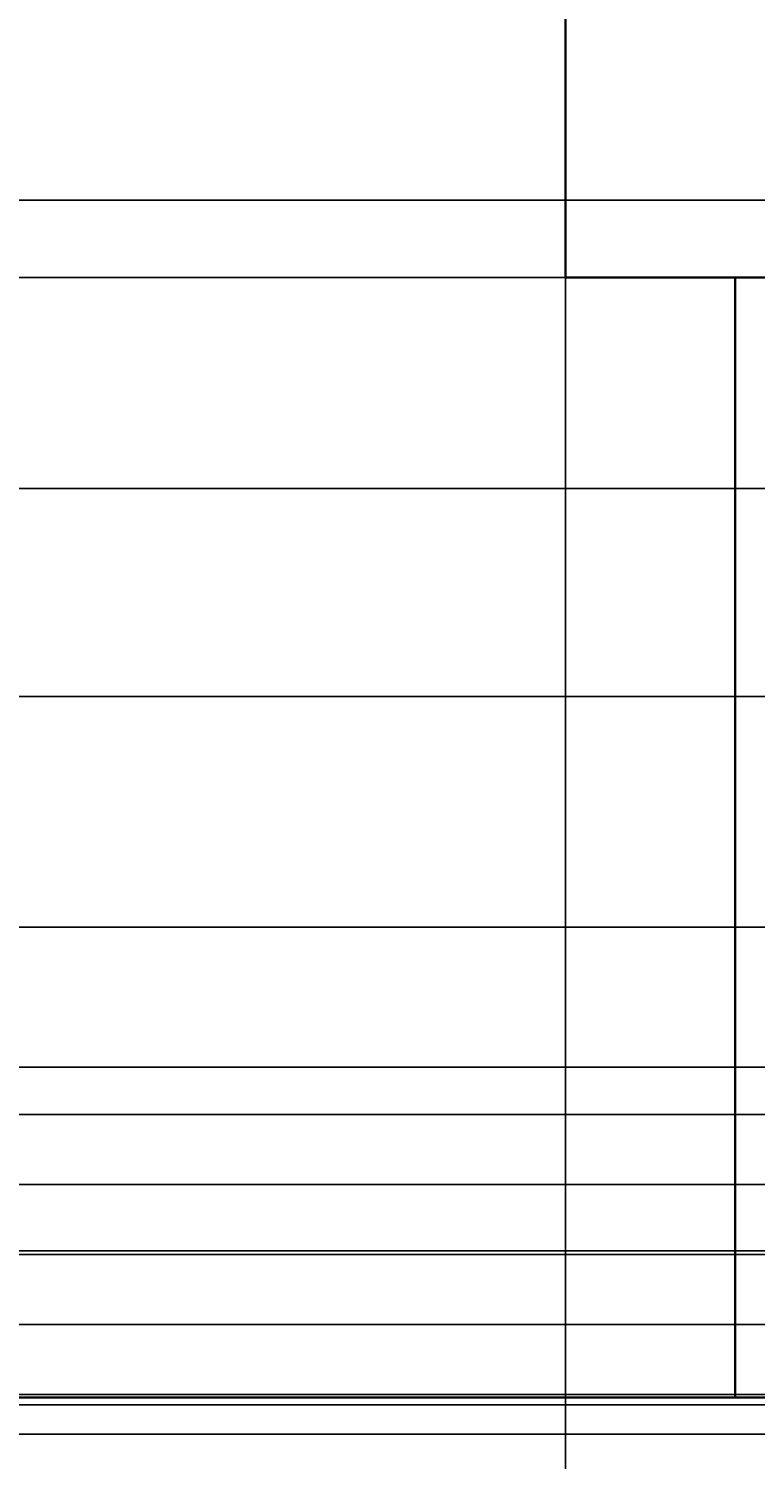
# Model space of a CAD drawing. Units: inches. Extents: x -13 to 809, y 112 to 656.
# Tile 4 of 55: x 49 to 111, y 205 to 328. Entities that reach past the tile are written whole.
import ezdxf

# ---------------------------------------------------------------- set-up
doc = ezdxf.new("R2010")
doc.units = ezdxf.units.IN
doc.header["$MEASUREMENT"] = 0
doc.layers.add('A-ANNO-DIMS', color=2, linetype='Continuous', lineweight=18)
doc.layers.add('A-ELEV', color=7, linetype='Continuous', lineweight=35)
doc.styles.get("Standard").update_dxf_attribs({"font": 'arial.ttf'})
doc.dimstyles.get("Standard").update_dxf_attribs({"dimtxt": 0.625, "dimasz": 0.18, "dimexe": 0.18, "dimexo": 0.0625, "dimgap": 0.09, "dimtad": 0, "dimtih": 1, "dimtoh": 1, "dimdec": 4, "dimzin": 0, "dimdsep": 46, "dimlunit": 4, "dimtxsty": 'Standard', "dimcen": 0.09, "dimadec": 0, "dimazin": 0, "dimtfac": 1, "dimtdec": 4, "dimtofl": 0, "dimtmove": 0, "dimatfit": 3, "dimfxl": 1, "dimtolj": 1, "dimtzin": 0, "dimarcsym": 0})

# ---------------------------------------------------------------- blocks, each defined once
blk = doc.blocks.new('*D11')
at = {"layer": 'A-ANNO-DIMS', "color": 0, "lineweight": -2, "transparency": 16777216}
for p, q in [((95.05, 306.46), (95.05, 112.34)), ((26.08, 150.46), (26.08, 112.34)), ((26.26, 112.52), (59.42, 112.52)), ((94.87, 112.52), (61.71, 112.52))]:
    blk.add_line(p, q, dxfattribs=at)
at = {"layer": 'A-ANNO-DIMS', "color": 0, "transparency": 16777216}
for points in [[(26.26, 112.55), (26.26, 112.49), (26.08, 112.52)], [(94.87, 112.55), (94.87, 112.49), (95.05, 112.52)]]:
    blk.add_solid(points, dxfattribs=at)
at = {"layer": 'Defpoints', "color": 0, "transparency": 16777216}
for p in [(95.05, 306.52), (26.08, 150.52), (95.05, 112.52)]:
    blk.add_point(p, dxfattribs=at)
at = {"layer": 'A-ANNO-DIMS', "color": 0, "transparency": 16777216, "insert": (60.56, 112.52), "char_height": 0.625, "attachment_point": 5}
blk.add_mtext('\\A1;68.97', dxfattribs=at)
blk = doc.blocks.new('*D12')
at = {"layer": 'A-ANNO-DIMS', "color": 0, "lineweight": -2, "transparency": 16777216}
for p, q in [((95.05, 306.46), (95.05, 112.34)), ((124.92, 210.46), (124.92, 112.34)), ((95.23, 112.52), (108.83, 112.52)), ((124.74, 112.52), (111.13, 112.52))]:
    blk.add_line(p, q, dxfattribs=at)
at = {"layer": 'A-ANNO-DIMS', "color": 0, "transparency": 16777216}
for points in [[(95.23, 112.55), (95.23, 112.49), (95.05, 112.52)], [(124.74, 112.55), (124.74, 112.49), (124.92, 112.52)]]:
    blk.add_solid(points, dxfattribs=at)
at = {"layer": 'Defpoints', "color": 0, "transparency": 16777216}
for p in [(95.05, 306.52), (124.92, 210.52), (124.92, 112.52)]:
    blk.add_point(p, dxfattribs=at)
at = {"layer": 'A-ANNO-DIMS', "color": 0, "transparency": 16777216, "insert": (109.98, 112.52), "char_height": 0.625, "attachment_point": 5}
blk.add_mtext('\\A1;29.87', dxfattribs=at)
blk = doc.blocks.new('*D22')
at = {"layer": 'A-ANNO-DIMS', "color": 0, "lineweight": -2, "transparency": 16777216}
for p, q in [((26.08, 210.58), (26.08, 655.96)), ((26.26, 655.78), (65.52, 655.78)), ((107.08, 655.78), (67.82, 655.78)), ((107.26, 510.58), (107.26, 655.96))]:
    blk.add_line(p, q, dxfattribs=at)
at = {"layer": 'A-ANNO-DIMS', "color": 0, "transparency": 16777216}
for points in [[(26.26, 655.81), (26.26, 655.75), (26.08, 655.78)], [(107.08, 655.81), (107.08, 655.75), (107.26, 655.78)]]:
    blk.add_solid(points, dxfattribs=at)
at = {"layer": 'Defpoints', "color": 0, "transparency": 16777216}
for p in [(107.26, 655.78), (107.26, 510.52), (26.08, 210.52)]:
    blk.add_point(p, dxfattribs=at)
at = {"layer": 'A-ANNO-DIMS', "color": 0, "transparency": 16777216, "insert": (66.67, 655.78), "char_height": 0.625, "attachment_point": 5}
blk.add_mtext('\\A1;81.18', dxfattribs=at)
blk = doc.blocks.new('*D33')
at = {"layer": 'A-ANNO-DIMS', "color": 0, "lineweight": -2, "transparency": 16777216}
for p, q in [((94.98, 306.52), (-12.1, 306.52)), ((-11.92, 306.34), (-11.92, 258.93)), ((-11.92, 210.7), (-11.92, 258.11)), ((26.02, 210.52), (-12.1, 210.52))]:
    blk.add_line(p, q, dxfattribs=at)
at = {"layer": 'A-ANNO-DIMS', "color": 0, "transparency": 16777216}
for points in [[(-11.95, 306.34), (-11.89, 306.34), (-11.92, 306.52)], [(-11.95, 210.7), (-11.89, 210.7), (-11.92, 210.52)]]:
    blk.add_solid(points, dxfattribs=at)
at = {"layer": 'Defpoints', "color": 0, "transparency": 16777216}
for p in [(-11.92, 306.52), (95.05, 306.52), (26.08, 210.52)]:
    blk.add_point(p, dxfattribs=at)
at = {"layer": 'A-ANNO-DIMS', "color": 0, "transparency": 16777216, "insert": (-11.92, 258.52), "char_height": 0.625, "attachment_point": 5}
blk.add_mtext('\\A1;96', dxfattribs=at)
blk = doc.blocks.new('*D34')
at = {"layer": 'A-ANNO-DIMS', "color": 0, "lineweight": -2, "transparency": 16777216}
for p, q in [((94.98, 462.52), (-12.1, 462.52)), ((-11.92, 462.34), (-11.92, 384.93)), ((-11.92, 306.7), (-11.92, 384.11)), ((94.98, 306.52), (-12.1, 306.52))]:
    blk.add_line(p, q, dxfattribs=at)
at = {"layer": 'A-ANNO-DIMS', "color": 0, "transparency": 16777216}
for points in [[(-11.95, 462.34), (-11.89, 462.34), (-11.92, 462.52)], [(-11.95, 306.7), (-11.89, 306.7), (-11.92, 306.52)]]:
    blk.add_solid(points, dxfattribs=at)
at = {"layer": 'Defpoints', "color": 0, "transparency": 16777216}
for p in [(-11.92, 462.52), (95.05, 462.52), (95.05, 306.52)]:
    blk.add_point(p, dxfattribs=at)
at = {"layer": 'A-ANNO-DIMS', "color": 0, "transparency": 16777216, "insert": (-11.92, 384.52), "char_height": 0.625, "attachment_point": 5}
blk.add_mtext('\\A1;156', dxfattribs=at)
blk = doc.blocks.new('*D39')
at = {"layer": 'A-ANNO-DIMS', "color": 0, "lineweight": -2, "transparency": 16777216}
for p, q in [((341.34, 524.28), (-12.1, 524.28)), ((-11.92, 524.1), (-11.92, 406.78)), ((-11.92, 288.63), (-11.92, 405.96)), ((341.34, 288.45), (-12.1, 288.45))]:
    blk.add_line(p, q, dxfattribs=at)
at = {"layer": 'A-ANNO-DIMS', "color": 0, "transparency": 16777216}
for points in [[(-11.95, 524.1), (-11.89, 524.1), (-11.92, 524.28)], [(-11.95, 288.63), (-11.89, 288.63), (-11.92, 288.45)]]:
    blk.add_solid(points, dxfattribs=at)
at = {"layer": 'Defpoints', "color": 0, "transparency": 16777216}
for p in [(-11.92, 524.28), (341.41, 524.28), (341.41, 288.45)]:
    blk.add_point(p, dxfattribs=at)
at = {"layer": 'A-ANNO-DIMS', "color": 0, "transparency": 16777216, "insert": (-11.92, 406.37), "char_height": 0.625, "attachment_point": 5}
blk.add_mtext('\\A1;235.83', dxfattribs=at)
blk = doc.blocks.new('*D40')
at = {"layer": 'A-ANNO-DIMS', "color": 0, "lineweight": -2, "transparency": 16777216}
for p, q in [((471.04, 313.17), (-12.1, 313.17)), ((-11.92, 312.99), (-11.92, 301.22)), ((-11.92, 288.63), (-11.92, 300.4)), ((341.34, 288.45), (-12.1, 288.45))]:
    blk.add_line(p, q, dxfattribs=at)
at = {"layer": 'A-ANNO-DIMS', "color": 0, "transparency": 16777216}
for points in [[(-11.95, 312.99), (-11.89, 312.99), (-11.92, 313.17)], [(-11.95, 288.63), (-11.89, 288.63), (-11.92, 288.45)]]:
    blk.add_solid(points, dxfattribs=at)
at = {"layer": 'Defpoints', "color": 0, "transparency": 16777216}
for p in [(471.1, 313.17), (-11.92, 288.45), (341.41, 288.45)]:
    blk.add_point(p, dxfattribs=at)
at = {"layer": 'A-ANNO-DIMS', "color": 0, "transparency": 16777216, "insert": (-11.92, 300.81), "char_height": 0.625, "attachment_point": 5}
blk.add_mtext('\\A1;24.716', dxfattribs=at)
blk = doc.blocks.new('*D41')
at = {"layer": 'A-ANNO-DIMS', "color": 0, "lineweight": -2, "transparency": 16777216}
for p, q in [((471.04, 357.98), (-12.1, 357.98)), ((-11.92, 357.8), (-11.92, 335.98)), ((-11.92, 313.35), (-11.92, 335.16)), ((471.04, 313.17), (-12.1, 313.17))]:
    blk.add_line(p, q, dxfattribs=at)
at = {"layer": 'A-ANNO-DIMS', "color": 0, "transparency": 16777216}
for points in [[(-11.95, 357.8), (-11.89, 357.8), (-11.92, 357.98)], [(-11.95, 313.35), (-11.89, 313.35), (-11.92, 313.17)]]:
    blk.add_solid(points, dxfattribs=at)
at = {"layer": 'Defpoints', "color": 0, "transparency": 16777216}
for p in [(-11.92, 357.98), (471.1, 357.98), (471.1, 313.17)]:
    blk.add_point(p, dxfattribs=at)
at = {"layer": 'A-ANNO-DIMS', "color": 0, "transparency": 16777216, "insert": (-11.92, 335.57), "char_height": 0.625, "attachment_point": 5}
blk.add_mtext('\\A1;44.81', dxfattribs=at)
blk = doc.blocks.new('*D44')
at = {"layer": 'A-ANNO-DIMS', "color": 0, "lineweight": -2, "transparency": 16777216}
for p, q in [((124.86, 270.6), (-12.1, 270.6)), ((-11.92, 270.42), (-11.92, 240.97)), ((-11.92, 210.7), (-11.92, 240.15)), ((124.86, 210.52), (-12.1, 210.52))]:
    blk.add_line(p, q, dxfattribs=at)
at = {"layer": 'A-ANNO-DIMS', "color": 0, "transparency": 16777216}
for points in [[(-11.95, 270.42), (-11.89, 270.42), (-11.92, 270.6)], [(-11.95, 210.7), (-11.89, 210.7), (-11.92, 210.52)]]:
    blk.add_solid(points, dxfattribs=at)
at = {"layer": 'Defpoints', "color": 0, "transparency": 16777216}
for p in [(-11.92, 270.6), (124.92, 270.6), (124.92, 210.52)]:
    blk.add_point(p, dxfattribs=at)
at = {"layer": 'A-ANNO-DIMS', "color": 0, "transparency": 16777216, "insert": (-11.92, 240.56), "char_height": 0.625, "attachment_point": 5}
blk.add_mtext('\\A1;60.08', dxfattribs=at)
blk = doc.blocks.new('*D45')
at = {"layer": 'A-ANNO-DIMS', "color": 0, "lineweight": -2, "transparency": 16777216}
for p, q in [((275.65, 270.6), (-12.1, 270.6)), ((-11.92, 270.42), (-11.92, 247.26)), ((-11.92, 223.28), (-11.92, 246.44)), ((275.65, 223.1), (-12.1, 223.1))]:
    blk.add_line(p, q, dxfattribs=at)
at = {"layer": 'A-ANNO-DIMS', "color": 0, "transparency": 16777216}
for points in [[(-11.95, 270.42), (-11.89, 270.42), (-11.92, 270.6)], [(-11.95, 223.28), (-11.89, 223.28), (-11.92, 223.1)]]:
    blk.add_solid(points, dxfattribs=at)
at = {"layer": 'Defpoints', "color": 0, "transparency": 16777216}
for p in [(-11.92, 270.6), (275.71, 270.6), (275.71, 223.1)]:
    blk.add_point(p, dxfattribs=at)
at = {"layer": 'A-ANNO-DIMS', "color": 0, "transparency": 16777216, "insert": (-11.92, 246.85), "char_height": 0.625, "attachment_point": 5}
blk.add_mtext('\\A1;47.5', dxfattribs=at)
blk = doc.blocks.new('*D49')
at = {"layer": 'A-ANNO-DIMS', "color": 0, "lineweight": -2, "transparency": 16777216}
for p, q in [((590.95, 250.84), (-12.1, 250.84)), ((-11.92, 250.66), (-11.92, 245.25)), ((-11.92, 239.02), (-11.92, 244.44)), ((590.95, 238.84), (-12.1, 238.84))]:
    blk.add_line(p, q, dxfattribs=at)
at = {"layer": 'A-ANNO-DIMS', "color": 0, "transparency": 16777216}
for points in [[(-11.95, 250.66), (-11.89, 250.66), (-11.92, 250.84)], [(-11.95, 239.02), (-11.89, 239.02), (-11.92, 238.84)]]:
    blk.add_solid(points, dxfattribs=at)
at = {"layer": 'Defpoints', "color": 0, "transparency": 16777216}
for p in [(-11.92, 250.84), (591.01, 250.84), (591.01, 238.84)]:
    blk.add_point(p, dxfattribs=at)
at = {"layer": 'A-ANNO-DIMS', "color": 0, "transparency": 16777216, "insert": (-11.92, 244.84), "char_height": 0.625, "attachment_point": 5}
blk.add_mtext('\\A1;12', dxfattribs=at)
blk = doc.blocks.new('*D50')
at = {"layer": 'A-ANNO-DIMS', "color": 0, "lineweight": -2, "transparency": 16777216}
for p, q in [((590.95, 238.84), (-12.1, 238.84)), ((-11.92, 238.66), (-11.92, 224.77)), ((-11.92, 210.06), (-11.92, 223.95)), ((607.51, 209.88), (-12.1, 209.88))]:
    blk.add_line(p, q, dxfattribs=at)
at = {"layer": 'A-ANNO-DIMS', "color": 0, "transparency": 16777216}
for points in [[(-11.95, 238.66), (-11.89, 238.66), (-11.92, 238.84)], [(-11.95, 210.06), (-11.89, 210.06), (-11.92, 209.88)]]:
    blk.add_solid(points, dxfattribs=at)
at = {"layer": 'Defpoints', "color": 0, "transparency": 16777216}
for p in [(591.01, 238.84), (-11.92, 209.88), (607.57, 209.88)]:
    blk.add_point(p, dxfattribs=at)
at = {"layer": 'A-ANNO-DIMS', "color": 0, "transparency": 16777216, "insert": (-11.92, 224.36), "char_height": 0.625, "attachment_point": 5}
blk.add_mtext('\\A1;28.97', dxfattribs=at)
blk = doc.blocks.new('*D80')
at = {"layer": 'A-ANNO-DIMS', "color": 0, "lineweight": -2, "transparency": 16777216}
for p, q in [((368.83, 216.77), (-12.1, 216.77)), ((-11.92, 216.59), (-11.92, 214.18)), ((-11.92, 210.95), (-11.92, 213.36)), ((368.83, 210.77), (-12.1, 210.77))]:
    blk.add_line(p, q, dxfattribs=at)
at = {"layer": 'A-ANNO-DIMS', "color": 0, "transparency": 16777216}
for points in [[(-11.95, 216.59), (-11.89, 216.59), (-11.92, 216.77)], [(-11.95, 210.95), (-11.89, 210.95), (-11.92, 210.77)]]:
    blk.add_solid(points, dxfattribs=at)
at = {"layer": 'Defpoints', "color": 0, "transparency": 16777216}
for p in [(-11.92, 216.77), (368.9, 216.77), (368.9, 210.77)]:
    blk.add_point(p, dxfattribs=at)
at = {"layer": 'A-ANNO-DIMS', "color": 0, "transparency": 16777216, "insert": (-11.92, 213.77), "char_height": 0.625, "attachment_point": 5}
blk.add_mtext('\\A1;6', dxfattribs=at)
blk = doc.blocks.new('*D81')
at = {"layer": 'A-ANNO-DIMS', "color": 0, "lineweight": -2, "transparency": 16777216}
for p, q in [((378.83, 222.77), (-12.1, 222.77)), ((-11.92, 222.59), (-11.92, 220.18)), ((-11.92, 216.95), (-11.92, 219.36)), ((378.83, 216.77), (-12.1, 216.77))]:
    blk.add_line(p, q, dxfattribs=at)
at = {"layer": 'A-ANNO-DIMS', "color": 0, "transparency": 16777216}
for points in [[(-11.95, 222.59), (-11.89, 222.59), (-11.92, 222.77)], [(-11.95, 216.95), (-11.89, 216.95), (-11.92, 216.77)]]:
    blk.add_solid(points, dxfattribs=at)
at = {"layer": 'Defpoints', "color": 0, "transparency": 16777216}
for p in [(-11.92, 222.77), (378.9, 222.77), (378.9, 216.77)]:
    blk.add_point(p, dxfattribs=at)
at = {"layer": 'A-ANNO-DIMS', "color": 0, "transparency": 16777216, "insert": (-11.92, 219.77), "char_height": 0.625, "attachment_point": 5}
blk.add_mtext('\\A1;6', dxfattribs=at)
blk = doc.blocks.new('*D82')
at = {"layer": 'A-ANNO-DIMS', "color": 0, "lineweight": -2, "transparency": 16777216}
for p, q in [((388.83, 228.77), (-12.1, 228.77)), ((-11.92, 228.59), (-11.92, 226.18)), ((-11.92, 222.95), (-11.92, 225.36)), ((388.83, 222.77), (-12.1, 222.77))]:
    blk.add_line(p, q, dxfattribs=at)
at = {"layer": 'A-ANNO-DIMS', "color": 0, "transparency": 16777216}
for points in [[(-11.95, 228.59), (-11.89, 228.59), (-11.92, 228.77)], [(-11.95, 222.95), (-11.89, 222.95), (-11.92, 222.77)]]:
    blk.add_solid(points, dxfattribs=at)
at = {"layer": 'Defpoints', "color": 0, "transparency": 16777216}
for p in [(-11.92, 228.77), (388.9, 228.77), (388.9, 222.77)]:
    blk.add_point(p, dxfattribs=at)
at = {"layer": 'A-ANNO-DIMS', "color": 0, "transparency": 16777216, "insert": (-11.92, 225.77), "char_height": 0.625, "attachment_point": 5}
blk.add_mtext('\\A1;6', dxfattribs=at)
blk = doc.blocks.new('*D83')
at = {"layer": 'A-ANNO-DIMS', "color": 0, "lineweight": -2, "transparency": 16777216}
for p, q in [((398.83, 234.77), (-12.1, 234.77)), ((-11.92, 234.59), (-11.92, 232.18)), ((-11.92, 228.95), (-11.92, 231.36)), ((398.83, 228.77), (-12.1, 228.77))]:
    blk.add_line(p, q, dxfattribs=at)
at = {"layer": 'A-ANNO-DIMS', "color": 0, "transparency": 16777216}
for points in [[(-11.95, 234.59), (-11.89, 234.59), (-11.92, 234.77)], [(-11.95, 228.95), (-11.89, 228.95), (-11.92, 228.77)]]:
    blk.add_solid(points, dxfattribs=at)
at = {"layer": 'Defpoints', "color": 0, "transparency": 16777216}
for p in [(-11.92, 234.77), (398.9, 234.77), (398.9, 228.77)]:
    blk.add_point(p, dxfattribs=at)
at = {"layer": 'A-ANNO-DIMS', "color": 0, "transparency": 16777216, "insert": (-11.92, 231.77), "char_height": 0.625, "attachment_point": 5}
blk.add_mtext('\\A1;6', dxfattribs=at)
blk = doc.blocks.new('*D84')
at = {"layer": 'A-ANNO-DIMS', "color": 0, "lineweight": -2, "transparency": 16777216}
for p, q in [((408.83, 238.84), (-12.1, 238.84)), ((-11.92, 238.66), (-11.92, 237.22)), ((-11.92, 234.95), (-11.92, 236.4)), ((408.83, 234.77), (-12.1, 234.77))]:
    blk.add_line(p, q, dxfattribs=at)
at = {"layer": 'A-ANNO-DIMS', "color": 0, "transparency": 16777216}
for points in [[(-11.95, 238.66), (-11.89, 238.66), (-11.92, 238.84)], [(-11.95, 234.95), (-11.89, 234.95), (-11.92, 234.77)]]:
    blk.add_solid(points, dxfattribs=at)
at = {"layer": 'Defpoints', "color": 0, "transparency": 16777216}
for p in [(-11.92, 238.84), (408.9, 238.84), (408.9, 234.77)]:
    blk.add_point(p, dxfattribs=at)
at = {"layer": 'A-ANNO-DIMS', "color": 0, "transparency": 16777216, "insert": (-11.92, 236.81), "char_height": 0.625, "attachment_point": 5}
blk.add_mtext('\\A1;4.069', dxfattribs=at)
blk = doc.blocks.new('*D90')
at = {"layer": 'A-ANNO-DIMS', "color": 0, "lineweight": -2, "transparency": 16777216}
for p, q in [((26.08, 210.46), (26.08, 112.34)), ((76.47, 195.83), (76.47, 112.34)), ((26.26, 112.52), (50.13, 112.52)), ((76.29, 112.52), (52.42, 112.52))]:
    blk.add_line(p, q, dxfattribs=at)
at = {"layer": 'A-ANNO-DIMS', "color": 0, "transparency": 16777216}
for points in [[(26.26, 112.55), (26.26, 112.49), (26.08, 112.52)], [(76.29, 112.55), (76.29, 112.49), (76.47, 112.52)]]:
    blk.add_solid(points, dxfattribs=at)
at = {"layer": 'Defpoints', "color": 0, "transparency": 16777216}
for p in [(26.08, 210.52), (76.47, 195.89), (76.47, 112.52)]:
    blk.add_point(p, dxfattribs=at)
at = {"layer": 'A-ANNO-DIMS', "color": 0, "transparency": 16777216, "insert": (51.28, 112.52), "char_height": 0.625, "attachment_point": 5}
blk.add_mtext('\\A1;50.39', dxfattribs=at)
blk = doc.blocks.new('*D94')
at = {"layer": 'A-ANNO-DIMS', "color": 0, "lineweight": -2, "transparency": 16777216}
for p, q in [((210.02, 223.1), (-12.1, 223.1)), ((-11.92, 222.92), (-11.92, 217.22)), ((-11.92, 210.7), (-11.92, 216.4)), ((160.86, 210.52), (-12.1, 210.52))]:
    blk.add_line(p, q, dxfattribs=at)
at = {"layer": 'A-ANNO-DIMS', "color": 0, "transparency": 16777216}
for points in [[(-11.95, 222.92), (-11.89, 222.92), (-11.92, 223.1)], [(-11.95, 210.7), (-11.89, 210.7), (-11.92, 210.52)]]:
    blk.add_solid(points, dxfattribs=at)
at = {"layer": 'Defpoints', "color": 0, "transparency": 16777216}
for p in [(-11.92, 223.1), (210.08, 223.1), (160.92, 210.52)]:
    blk.add_point(p, dxfattribs=at)
at = {"layer": 'A-ANNO-DIMS', "color": 0, "transparency": 16777216, "insert": (-11.92, 216.81), "char_height": 0.625, "attachment_point": 5}
blk.add_mtext('\\A1;12.58', dxfattribs=at)
blk = doc.blocks.new('*D107')
at = {"layer": 'A-ANNO-DIMS', "color": 0, "lineweight": -2, "transparency": 16777216}
for p, q in [((113.05, 324.46), (113.05, 112.34)), ((95.05, 306.46), (95.05, 112.34)), ((95.23, 112.52), (102.93, 112.52)), ((112.87, 112.52), (105.16, 112.52))]:
    blk.add_line(p, q, dxfattribs=at)
at = {"layer": 'A-ANNO-DIMS', "color": 0, "transparency": 16777216}
for points in [[(95.23, 112.55), (95.23, 112.49), (95.05, 112.52)], [(112.87, 112.55), (112.87, 112.49), (113.05, 112.52)]]:
    blk.add_solid(points, dxfattribs=at)
at = {"layer": 'Defpoints', "color": 0, "transparency": 16777216}
for p in [(113.05, 324.52), (95.05, 306.52), (113.05, 112.52)]:
    blk.add_point(p, dxfattribs=at)
at = {"layer": 'A-ANNO-DIMS', "color": 0, "transparency": 16777216, "insert": (104.05, 112.52), "char_height": 0.625, "attachment_point": 5}
blk.add_mtext('\\A1;18.00', dxfattribs=at)
blk = doc.blocks.new('*D115')
at = {"layer": 'A-ANNO-DIMS', "color": 0, "lineweight": -2, "transparency": 16777216}
for p, q in [((311.4, 210.78), (-12.1, 210.78)), ((-11.92, 210.6), (-11.92, 181.06)), ((-11.92, 150.7), (-11.92, 180.24)), ((311.64, 150.52), (-12.1, 150.52))]:
    blk.add_line(p, q, dxfattribs=at)
at = {"layer": 'A-ANNO-DIMS', "color": 0, "transparency": 16777216}
for points in [[(-11.95, 210.6), (-11.89, 210.6), (-11.92, 210.78)], [(-11.95, 150.7), (-11.89, 150.7), (-11.92, 150.52)]]:
    blk.add_solid(points, dxfattribs=at)
at = {"layer": 'Defpoints', "color": 0, "transparency": 16777216}
for p in [(-11.92, 210.78), (311.46, 210.78), (311.7, 150.52)]:
    blk.add_point(p, dxfattribs=at)
at = {"layer": 'A-ANNO-DIMS', "color": 0, "transparency": 16777216, "insert": (-11.92, 180.65), "char_height": 0.625, "attachment_point": 5}
blk.add_mtext('\\A1;60.27', dxfattribs=at)
blk = doc.blocks.new('*D118')
at = {"layer": 'A-ANNO-DIMS', "color": 0, "lineweight": -2, "transparency": 16777216}
for p, q in [((311.4, 210.78), (-12.1, 210.78)), ((-11.92, 210.6), (-11.92, 209.49)), ((-11.92, 207.55), (-11.92, 208.67)), ((308.59, 207.37), (-12.1, 207.37))]:
    blk.add_line(p, q, dxfattribs=at)
at = {"layer": 'A-ANNO-DIMS', "color": 0, "transparency": 16777216}
for points in [[(-11.95, 210.6), (-11.89, 210.6), (-11.92, 210.78)], [(-11.95, 207.55), (-11.89, 207.55), (-11.92, 207.37)]]:
    blk.add_solid(points, dxfattribs=at)
at = {"layer": 'Defpoints', "color": 0, "transparency": 16777216}
for p in [(-11.92, 210.78), (311.46, 210.78), (308.65, 207.37)]:
    blk.add_point(p, dxfattribs=at)
at = {"layer": 'A-ANNO-DIMS', "color": 0, "transparency": 16777216, "insert": (-11.92, 209.08), "char_height": 0.625, "attachment_point": 5}
blk.add_mtext('\\A1;3.41', dxfattribs=at)

msp = doc.modelspace()

# ---------------------------------------------------------------- linework, layer by layer
at = {"layer": 'A-ELEV'}
for p, q in [((95.0469, 318.5199), (95.0469, 462.5199)), ((95.0469, 306.5199), (95.0469, 318.5199)), ((109.5888, 306.5199), (95.0469, 306.5199)), ((109.5888, 210.5199), (109.5888, 306.5199)), ((109.5888, 306.5199), (337.5074, 306.5199)), ((26.0809, 210.5199), (256.4464, 210.5199))]:
    msp.add_line(p, q, dxfattribs=at)

# ---------------------------------------------------------------- dimensions: what is measured, and where the dimension line sits
at = {"layer": 'A-ANNO-DIMS'}
for base, p1, p2, picture, middle in [((107.2588, 655.7828), (26.0809, 210.5199), (107.2588, 510.5199), '*D22', (66.6698, 655.7828)), ((113.0469, 112.5199), (95.0469, 306.5199), (113.0469, 324.5199), '*D107', (104.0469, 112.5199)), ((95.0469, 112.5199), (26.0809, 150.5199), (95.0469, 306.5199), '*D11', (60.5639, 112.5199)), ((124.9184, 112.5199), (95.0469, 306.5199), (124.9184, 210.5199), '*D12', (109.9827, 112.5199)), ((76.4733, 112.5199), (26.0809, 210.5199), (76.4733, 195.8907), '*D90', (51.2771, 112.5199))]:
    dim = msp.add_linear_dim(base=base, p1=p1, p2=p2, dimstyle='Standard', override={"dimdec": 2, "dimlfac": 1, "dimrnd": 0, "dimzin": 0, "dimdsep": 46, "dimlunit": 2}, dxfattribs=at)
    dim.commit()
    dim.dimension.update_dxf_attribs({"geometry": picture, "text_midpoint": middle})
for base, p1, p2, override, picture, middle in [((-11.9191, 524.281), (341.4072, 288.4508), (341.4072, 524.281), {"dimdec": 2, "dimlfac": 1, "dimrnd": 0, "dimzin": 0, "dimdsep": 46, "dimlunit": 2}, '*D39', (-11.9191, 406.3659)), ((-11.9191, 462.5199), (95.0469, 306.5199), (95.0469, 462.5199), {"dimdec": 0, "dimlfac": 1, "dimrnd": 0, "dimzin": 0, "dimdsep": 46, "dimlunit": 2}, '*D34', (-11.9191, 384.5199)), ((-11.9191, 357.9804), (471.0998, 313.1667), (471.0998, 357.9804), {"dimdec": 2, "dimlfac": 1, "dimrnd": 0, "dimzin": 0, "dimdsep": 46, "dimlunit": 2}, '*D41', (-11.9191, 335.5735)), ((-11.9191, 288.4508), (471.0998, 313.1667), (341.4072, 288.4508), {"dimdec": 3, "dimlfac": 1, "dimrnd": 0, "dimzin": 0, "dimdsep": 46, "dimlunit": 2}, '*D40', (-11.9191, 300.8087)), ((-11.9191, 306.5199), (26.0809, 210.5199), (95.0469, 306.5199), {"dimdec": 0, "dimlfac": 1, "dimrnd": 0, "dimzin": 0, "dimdsep": 46, "dimlunit": 2}, '*D33', (-11.9191, 258.5199)), ((-11.9191, 270.6024), (124.9184, 210.5199), (124.9184, 270.6024), {"dimdec": 2, "dimlfac": 1, "dimrnd": 0, "dimzin": 0, "dimdsep": 46, "dimlunit": 2}, '*D44', (-11.9191, 240.5611)), ((-11.9191, 270.6024), (275.7145, 223.1), (275.7145, 270.6024), {"dimdec": 1, "dimlfac": 1, "dimrnd": 0, "dimzin": 0, "dimdsep": 46, "dimlunit": 2}, '*D45', (-11.9191, 246.8512)), ((-11.9191, 250.8429), (591.008, 238.8429), (591.008, 250.8429), {"dimdec": 0, "dimlfac": 1, "dimrnd": 0, "dimzin": 0, "dimdsep": 46, "dimlunit": 2}, '*D49', (-11.9191, 244.8429)), ((-11.9191, 209.8753), (591.008, 238.8429), (607.5741, 209.8753), {"dimdec": 2, "dimlfac": 1, "dimrnd": 0, "dimzin": 0, "dimdsep": 46, "dimlunit": 2}, '*D50', (-11.9191, 224.3591)), ((-11.9191, 238.8429), (408.8966, 234.7738), (408.8966, 238.8429), {"dimdec": 3, "dimlfac": 1, "dimrnd": 0, "dimzin": 0, "dimdsep": 46, "dimlunit": 2}, '*D84', (-11.9191, 236.8083)), ((-11.9191, 234.7738), (398.8966, 228.7738), (398.8966, 234.7738), {"dimdec": 0, "dimlfac": 1, "dimrnd": 0, "dimzin": 0, "dimdsep": 46, "dimlunit": 2}, '*D83', (-11.9191, 231.7738)), ((-11.9191, 228.7738), (388.8966, 222.7738), (388.8966, 228.7738), {"dimdec": 0, "dimlfac": 1, "dimrnd": 0, "dimzin": 0, "dimdsep": 46, "dimlunit": 2}, '*D82', (-11.9191, 225.7738)), ((-11.9191, 223.1), (160.9184, 210.5199), (210.0791, 223.1), {"dimdec": 2, "dimlfac": 1, "dimrnd": 0, "dimzin": 0, "dimdsep": 46, "dimlunit": 2}, '*D94', (-11.9191, 216.81)), ((-11.9191, 222.7738), (378.8966, 216.7738), (378.8966, 222.7738), {"dimdec": 0, "dimlfac": 1, "dimrnd": 0, "dimzin": 0, "dimdsep": 46, "dimlunit": 2}, '*D81', (-11.9191, 219.7738)), ((-11.9191, 216.7738), (368.8966, 210.7738), (368.8966, 216.7738), {"dimdec": 0, "dimlfac": 1, "dimrnd": 0, "dimzin": 0, "dimdsep": 46, "dimlunit": 2}, '*D80', (-11.9191, 213.7738)), ((-11.91915, 210.78493), (311.6991, 150.51989), (311.46269, 210.78493), {"dimdec": 2, "dimlfac": 1, "dimrnd": 0, "dimzin": 0, "dimdsep": 46, "dimlunit": 2}, '*D115', (-11.91915, 180.65241)), ((-11.9191, 210.7849), (308.6488, 207.3724), (311.4627, 210.7849), {"dimdec": 2, "dimlfac": 1, "dimrnd": 0, "dimzin": 0, "dimdsep": 46, "dimlunit": 2}, '*D118', (-11.9191, 209.0787))]:
    dim = msp.add_linear_dim(base=base, p1=p1, p2=p2, angle=90, dimstyle='Standard', override=override, dxfattribs=at)
    dim.commit()
    dim.dimension.update_dxf_attribs({"geometry": picture, "text_midpoint": middle})

doc.saveas('drawing.dxf')
